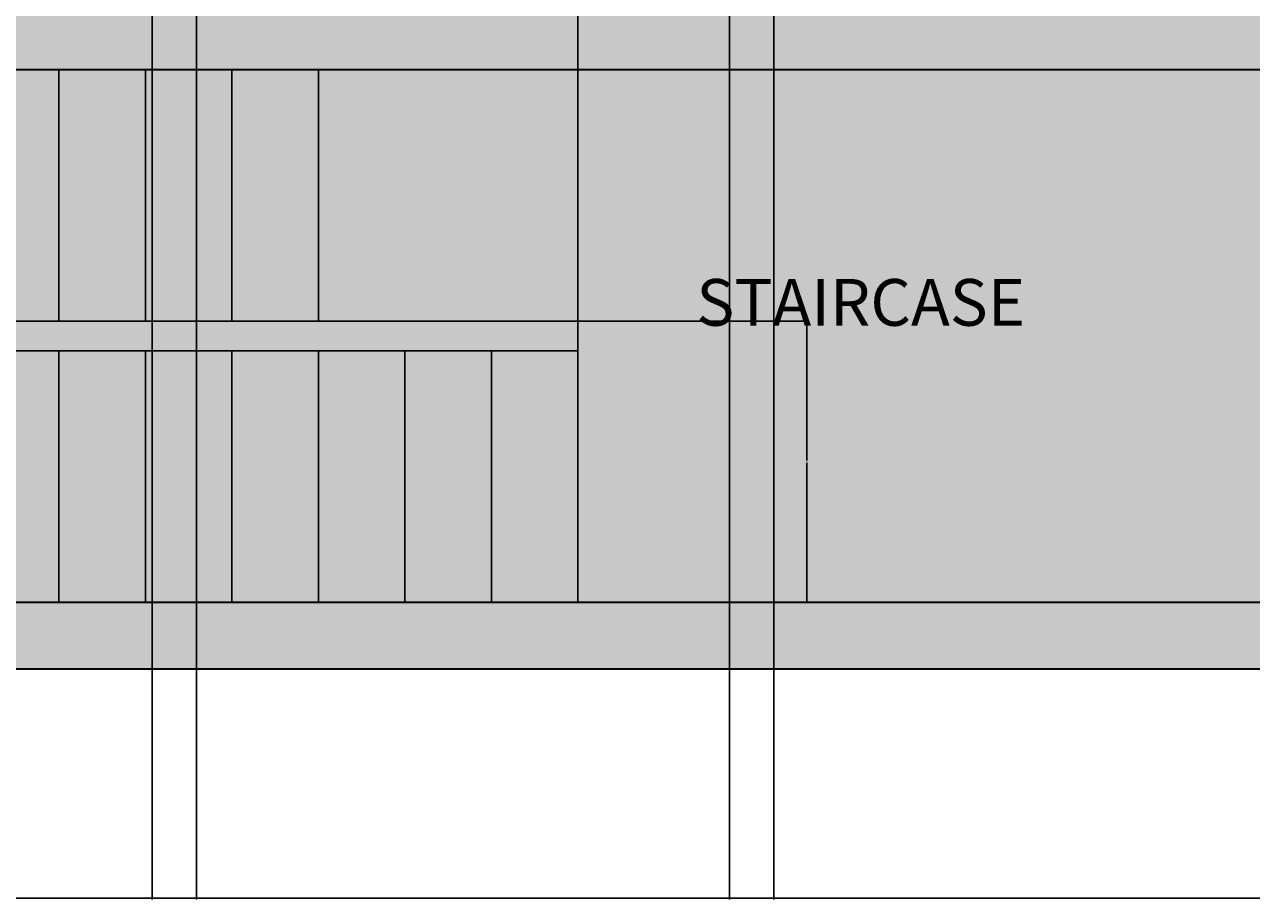
# Model space of a CAD drawing. Units: inches. Extents: x 2549 to 3108, y 1683 to 2362.
# Tile 2 of 30: x 2711 to 2877, y 1683 to 1802. Entities that reach past the tile are written whole.
import ezdxf

# ---------------------------------------------------------------- set-up
doc = ezdxf.new("R2010")
doc.units = ezdxf.units.IN
for name, color, linetype, lineweight in [('A-ANNO-DIMS', 2, 'Continuous', 18), ('A-AREA-IDEN', 7, 'Continuous', 18), ('A-FLOR-STRS', 7, 'Continuous', 25), ('A-FLOR-STRS-PATT', 41, 'Continuous', 13), ('A-FURN-PATT', 9, 'Continuous', 13), ('A-WALL', 7, 'Continuous', 35), ('A-WALL-PATT', 89, 'Continuous', 13), ('C-PROP', 7, 'Continuous', 35)]:
    doc.layers.add(name, color=color, linetype=linetype, lineweight=lineweight)
for name, color, linetype, lineweight, true_color in [('C-PKNG-VEHI-PATT', 251, 'Continuous', 13, 0x636466), ('C-PROP-PATT', 252, 'Continuous', 13, 0x939598), ('C-PVMT-PATT', 9, 'Continuous', 13, 0xc7c8ca)]:
    doc.layers.add(name, color=color, linetype=linetype, lineweight=lineweight, true_color=true_color)
doc.styles.get("Standard").update_dxf_attribs({"font": 'arial.ttf'})
doc.dimstyles.get("Standard").update_dxf_attribs({"dimtxt": 0.18, "dimasz": 0.18, "dimexe": 0.18, "dimexo": 0.0625, "dimgap": 0.09, "dimtad": 0, "dimtih": 1, "dimtoh": 1, "dimdec": 4, "dimzin": 0, "dimdsep": 46, "dimtxsty": 'Standard', "dimcen": 0.09, "dimadec": 0, "dimazin": 0, "dimtfac": 1, "dimtdec": 4, "dimtofl": 0, "dimtmove": 0, "dimatfit": 3, "dimfxl": 1, "dimtolj": 1, "dimtzin": 0, "dimarcsym": 0})

# ---------------------------------------------------------------- blocks, each defined once
blk = doc.blocks.new('*D24')
at = {"layer": 'A-ANNO-DIMS', "color": 0, "lineweight": -2, "transparency": 16777216}
for p, q in [((2596.64, 1714.46), (2596.64, 1683.44)), ((3076.64, 1714.46), (3076.64, 1683.44)), ((2596.82, 1683.62), (2836.35, 1683.62)), ((3076.46, 1683.62), (2836.93, 1683.62))]:
    blk.add_line(p, q, dxfattribs=at)
at = {"layer": 'A-ANNO-DIMS', "color": 0, "transparency": 16777216}
for points in [[(2596.82, 1683.65), (2596.82, 1683.59), (2596.64, 1683.62)], [(3076.46, 1683.65), (3076.46, 1683.59), (3076.64, 1683.62)]]:
    blk.add_solid(points, dxfattribs=at)
at = {"layer": 'Defpoints', "color": 0, "transparency": 16777216}
for p in [(2596.64, 1714.52), (3076.64, 1714.52), (3076.64, 1683.62)]:
    blk.add_point(p, dxfattribs=at)
at = {"layer": 'A-ANNO-DIMS', "color": 0, "transparency": 16777216, "insert": (2836.64, 1683.62), "char_height": 0.18, "attachment_point": 5}
blk.add_mtext('\\A1;480', dxfattribs=at)
blk = doc.blocks.new('*D42')
at = {"layer": 'A-ANNO-DIMS', "color": 0, "lineweight": -2, "transparency": 16777216}
for p, q in [((2638.64, 2080.46), (2638.64, 1683.44)), ((2728.64, 2080.46), (2728.64, 1683.44)), ((2638.82, 1683.62), (2683.42, 1683.62)), ((2728.46, 1683.62), (2683.86, 1683.62))]:
    blk.add_line(p, q, dxfattribs=at)
at = {"layer": 'A-ANNO-DIMS', "color": 0, "transparency": 16777216}
for points in [[(2638.82, 1683.65), (2638.82, 1683.59), (2638.64, 1683.62)], [(2728.46, 1683.65), (2728.46, 1683.59), (2728.64, 1683.62)]]:
    blk.add_solid(points, dxfattribs=at)
at = {"layer": 'Defpoints', "color": 0, "transparency": 16777216}
for p in [(2638.64, 2080.52), (2728.64, 2080.52), (2728.64, 1683.62)]:
    blk.add_point(p, dxfattribs=at)
at = {"layer": 'A-ANNO-DIMS', "color": 0, "transparency": 16777216, "insert": (2683.64, 1683.62), "char_height": 0.18, "attachment_point": 5}
blk.add_mtext('\\A1;90', dxfattribs=at)
blk = doc.blocks.new('*D43')
at = {"layer": 'A-ANNO-DIMS', "color": 0, "lineweight": -2, "transparency": 16777216}
for p, q in [((2734.64, 2080.46), (2734.64, 1683.44)), ((2806.64, 2080.46), (2806.64, 1683.44)), ((2734.82, 1683.62), (2770.43, 1683.62)), ((2806.46, 1683.62), (2770.86, 1683.62))]:
    blk.add_line(p, q, dxfattribs=at)
at = {"layer": 'A-ANNO-DIMS', "color": 0, "transparency": 16777216}
for points in [[(2734.82, 1683.65), (2734.82, 1683.59), (2734.64, 1683.62)], [(2806.46, 1683.65), (2806.46, 1683.59), (2806.64, 1683.62)]]:
    blk.add_solid(points, dxfattribs=at)
at = {"layer": 'Defpoints', "color": 0, "transparency": 16777216}
for p in [(2734.64, 2080.52), (2806.64, 2080.52), (2806.64, 1683.62)]:
    blk.add_point(p, dxfattribs=at)
at = {"layer": 'A-ANNO-DIMS', "color": 0, "transparency": 16777216, "insert": (2770.64, 1683.62), "char_height": 0.18, "attachment_point": 5}
blk.add_mtext('\\A1;72', dxfattribs=at)
blk = doc.blocks.new('*D44')
at = {"layer": 'A-ANNO-DIMS', "color": 0, "lineweight": -2, "transparency": 16777216}
for p, q in [((2662.64, 2040.99), (2662.64, 1683.44)), ((2806.64, 2016.13), (2806.64, 1683.44)), ((2662.82, 1683.62), (2734.36, 1683.62)), ((2806.46, 1683.62), (2734.92, 1683.62))]:
    blk.add_line(p, q, dxfattribs=at)
at = {"layer": 'A-ANNO-DIMS', "color": 0, "transparency": 16777216}
for points in [[(2662.82, 1683.65), (2662.82, 1683.59), (2662.64, 1683.62)], [(2806.46, 1683.65), (2806.46, 1683.59), (2806.64, 1683.62)]]:
    blk.add_solid(points, dxfattribs=at)
at = {"layer": 'Defpoints', "color": 0, "transparency": 16777216}
for p in [(2662.64, 2041.06), (2806.64, 2016.19), (2806.64, 1683.62)]:
    blk.add_point(p, dxfattribs=at)
at = {"layer": 'A-ANNO-DIMS', "color": 0, "transparency": 16777216, "insert": (2734.64, 1683.62), "char_height": 0.18, "attachment_point": 5}
blk.add_mtext('\\A1;144', dxfattribs=at)
blk = doc.blocks.new('*D46')
at = {"layer": 'A-ANNO-DIMS', "color": 0, "lineweight": -2, "transparency": 16777216}
for p, q in [((2812.64, 2140.46), (2812.64, 1683.44)), ((3034.64, 2134.46), (3034.64, 1683.44)), ((2812.82, 1683.62), (2923.35, 1683.62)), ((3034.46, 1683.62), (2923.93, 1683.62))]:
    blk.add_line(p, q, dxfattribs=at)
at = {"layer": 'A-ANNO-DIMS', "color": 0, "transparency": 16777216}
for points in [[(2812.82, 1683.65), (2812.82, 1683.59), (2812.64, 1683.62)], [(3034.46, 1683.65), (3034.46, 1683.59), (3034.64, 1683.62)]]:
    blk.add_solid(points, dxfattribs=at)
at = {"layer": 'Defpoints', "color": 0, "transparency": 16777216}
for p in [(2812.64, 2140.52), (3034.64, 2134.52), (3034.64, 1683.62)]:
    blk.add_point(p, dxfattribs=at)
at = {"layer": 'A-ANNO-DIMS', "color": 0, "transparency": 16777216, "insert": (2923.64, 1683.62), "char_height": 0.18, "attachment_point": 5}
blk.add_mtext('\\A1;222', dxfattribs=at)
blk = doc.blocks.new('*D59')
at = {"layer": 'A-ANNO-DIMS', "color": 0, "lineweight": -2, "transparency": 16777216}
for p, q in [((2680.98, 1761.59), (2680.98, 2362.32)), ((2681.16, 2362.14), (2733.11, 2362.14)), ((2785.98, 2362.14), (2734.02, 2362.14)), ((2786.16, 1761.59), (2786.16, 2362.32))]:
    blk.add_line(p, q, dxfattribs=at)
at = {"layer": 'A-ANNO-DIMS', "color": 0, "transparency": 16777216}
for points in [[(2681.16, 2362.17), (2681.16, 2362.11), (2680.98, 2362.14)], [(2785.98, 2362.17), (2785.98, 2362.11), (2786.16, 2362.14)]]:
    blk.add_solid(points, dxfattribs=at)
at = {"layer": 'Defpoints', "color": 0, "transparency": 16777216}
for p in [(2786.16, 2362.14), (2680.98, 1761.52), (2786.16, 1761.52)]:
    blk.add_point(p, dxfattribs=at)
at = {"layer": 'A-ANNO-DIMS', "color": 0, "transparency": 16777216, "insert": (2733.57, 2362.14), "char_height": 0.18, "attachment_point": 5}
blk.add_mtext('\\A1;105.18', dxfattribs=at)
blk = doc.blocks.new('*D60')
at = {"layer": 'A-ANNO-DIMS', "color": 0, "lineweight": -2, "transparency": 16777216}
for p, q in [((2786.22, 1761.52), (2817.24, 1761.52)), ((2817.06, 1761.34), (2817.06, 1742.71)), ((2817.06, 1723.7), (2817.06, 1742.34)), ((2786.22, 1723.52), (2817.24, 1723.52))]:
    blk.add_line(p, q, dxfattribs=at)
at = {"layer": 'A-ANNO-DIMS', "color": 0, "transparency": 16777216}
for points in [[(2817.03, 1761.34), (2817.09, 1761.34), (2817.06, 1761.52)], [(2817.03, 1723.7), (2817.09, 1723.7), (2817.06, 1723.52)]]:
    blk.add_solid(points, dxfattribs=at)
at = {"layer": 'Defpoints', "color": 0, "transparency": 16777216}
for p in [(2786.16, 1761.52), (2786.16, 1723.52), (2817.06, 1723.52)]:
    blk.add_point(p, dxfattribs=at)
at = {"layer": 'A-ANNO-DIMS', "color": 0, "transparency": 16777216, "insert": (2817.06, 1742.52), "char_height": 0.18, "attachment_point": 5}
blk.add_mtext('\\A1;38', dxfattribs=at)

msp = doc.modelspace()

# ---------------------------------------------------------------- hatches: boundary and pattern name
at = {"layer": 'A-FLOR-STRS-PATT', "transparency": 33554567}
h = msp.add_hatch(color=256, dxfattribs=at)
h.dxf.hatch_style = 1
h.paths.add_polyline_path([(2680.9778, 1795.5237), (2662.6427, 1795.5237), (2638.6427, 1795.5237), (2638.6427, 1723.5237), (2680.9778, 1723.5237)])
h.paths.add_polyline_path([(2692.6645, 1795.5237), (2680.9778, 1795.5237), (2680.9778, 1761.5237), (2692.6645, 1761.5237)])
h.paths.add_polyline_path([(2704.3511, 1795.5237), (2692.6645, 1795.5237), (2692.6645, 1761.5237), (2704.3511, 1761.5237)])
h.paths.add_polyline_path([(2716.0378, 1795.5237), (2704.3511, 1795.5237), (2704.3511, 1761.5237), (2716.0378, 1761.5237)])
h.paths.add_polyline_path([(2727.7244, 1795.5237), (2716.0378, 1795.5237), (2716.0378, 1761.5237), (2727.7244, 1761.5237)])
h.paths.add_polyline_path([(2739.4111, 1795.5237), (2727.7244, 1795.5237), (2727.7244, 1761.5237), (2739.4111, 1761.5237)])
h.paths.add_polyline_path([(2751.0977, 1795.5237), (2739.4111, 1795.5237), (2739.4111, 1761.5237), (2751.0977, 1761.5237)])
h.paths.add_polyline_path([(2786.1577, 1757.5237), (2774.471, 1757.5237), (2774.471, 1723.5237), (2786.1577, 1723.5237)])
h.paths.add_polyline_path([(2774.471, 1757.5237), (2762.7844, 1757.5237), (2762.7844, 1723.5237), (2774.471, 1723.5237)])
h.paths.add_polyline_path([(2762.7844, 1757.5237), (2751.0977, 1757.5237), (2751.0977, 1723.5237), (2762.7844, 1723.5237)])
h.paths.add_polyline_path([(2751.0977, 1757.5237), (2739.4111, 1757.5237), (2739.4111, 1723.5237), (2751.0977, 1723.5237)])
h.paths.add_polyline_path([(2727.7244, 1757.5237), (2716.0378, 1757.5237), (2716.0378, 1723.5237), (2727.7244, 1723.5237)])
h.paths.add_polyline_path([(2716.0378, 1757.5237), (2704.3511, 1757.5237), (2704.3511, 1723.5237), (2716.0378, 1723.5237)])
h.paths.add_polyline_path([(2704.3511, 1757.5237), (2692.6645, 1757.5237), (2692.6645, 1723.5237), (2704.3511, 1723.5237)])
h.paths.add_polyline_path([(2692.6645, 1757.5237), (2680.9778, 1757.5237), (2680.9778, 1723.5237), (2692.6645, 1723.5237)])
h.paths.add_polyline_path([(2739.4111, 1757.5237), (2727.7244, 1757.5237), (2727.7244, 1723.5237), (2739.4111, 1723.5237)])
h.paths.add_polyline_path([(2786.1577, 1761.5237), (2680.9778, 1761.5237), (2680.9778, 1757.5237), (2786.1577, 1757.5237)])
at = {"layer": 'A-FURN-PATT', "transparency": 33554567}
h = msp.add_hatch(color=256, dxfattribs=at)
h.dxf.hatch_style = 1
h.paths.add_polyline_path([(2708.7147, 2271.6737), (2675.2813, 2271.6737), (2675.2813, 2262.0404), (2708.7147, 2262.0404)])
h.paths.add_polyline_path([(2980.8246, 2271.6737), (2947.3913, 2271.6737), (2947.3913, 2262.0404), (2980.8246, 2262.0404)])
h.paths.add_polyline_path([(2748.8496, 2101.6383), (2798.148, 2101.6383), (2798.148, 2111.4248), (2748.8496, 2111.4248)], flags=9)
h.paths.add_polyline_path([(2685.2081, 2101.489), (2719.3253, 2101.489), (2719.3253, 2111.2819), (2685.2081, 2111.2819)], flags=9)
h.paths.add_polyline_path([(2814.6852, 1907.1328), (2847.8384, 1907.1328), (2847.8384, 1916.9258), (2814.6852, 1916.9258)], flags=9)
h.paths.add_polyline_path([(2814.3906, 1835.5864), (2848.0172, 1835.5864), (2848.0172, 1845.3794), (2814.3906, 1845.3794)], flags=9)
h.paths.add_polyline_path([(2800.5245, 1759.1674), (2853.7435, 1759.1674), (2853.7435, 1768.954), (2800.5245, 1768.954)], flags=9)
h.paths.add_polyline_path([(2972.4611, 1807.3305), (3015.3943, 1807.3305), (3015.3943, 1817.117), (2972.4611, 1817.117)], flags=9)
h.paths.add_polyline_path([(2902.3327, 1888.6731), (2937.9131, 1888.6731), (2937.9131, 1898.4661), (2902.3327, 1898.4661)], flags=9)
h.paths.add_polyline_path([(2712.1779, 1878.9039), (2754.1257, 1878.9039), (2754.1257, 1888.6904), (2712.1779, 1888.6904)], flags=9)
h.paths.add_polyline_path([(2614.0056, 2012.812), (2650.0251, 2012.812), (2650.0251, 2022.4371), (2614.0056, 2022.4371)], flags=9)
h.paths.add_polyline_path([(2713.3129, 2003.1645), (2747.4237, 2003.1645), (2747.4237, 2012.951), (2713.3129, 2012.951)], flags=9)
h.paths.add_polyline_path([(2950.1379, 2001.6934), (2982.2992, 2001.6934), (2982.2992, 2011.48), (2950.1379, 2011.48)], flags=9)
h.paths.add_polyline_path([(2940.864, 2238.5537), (2997.5066, 2238.5537), (2997.5066, 2248.3466), (2940.864, 2248.3466)], flags=9)
h.paths.add_polyline_path([(2821.5457, 2202.8348), (2855.663, 2202.8348), (2855.663, 2212.6278), (2821.5457, 2212.6278)], flags=9)
h.paths.add_polyline_path([(2661.8026, 2238.6249), (2718.4451, 2238.6249), (2718.4451, 2248.4179), (2661.8026, 2248.4179)], flags=9)
h = msp.add_hatch(color=256, dxfattribs=at)
h.dxf.hatch_style = 1
h.paths.add_polyline_path([(2906.5064, 1905.2148), (2905.2584, 1904.3827), (2907.0611, 1900.7772), (2908.3092, 1901.6092)])
h.paths.add_polyline_path([(2936.522, 1914.8044), (2935.2739, 1915.6364), (2932.6391, 1912.5856), (2933.8871, 1911.7535)])
h.paths.add_polyline_path([(2950.2508, 1905.6518), (2949.0027, 1906.4839), (2947.1999, 1902.8783), (2948.448, 1902.0463)])
h.paths.add_polyline_path([(2958.5713, 1918.1326), (2956.9072, 1919.242), (2952.4696, 1908.98, 1.38742744), (2954.9657, 1907.3159)])
h.paths.add_polyline_path([(2945.2585, 1927.0078), (2943.5944, 1928.1172), (2934.9965, 1920.6287, 1.38742744), (2937.4927, 1918.9646)])
h.paths.add_polyline_path([(2748.8496, 2101.6383), (2798.148, 2101.6383), (2798.148, 2111.4248), (2748.8496, 2111.4248)], flags=9)
h.paths.add_polyline_path([(2685.2081, 2101.489), (2719.3253, 2101.489), (2719.3253, 2111.2819), (2685.2081, 2111.2819)], flags=9)
h.paths.add_polyline_path([(2814.6852, 1907.1328), (2847.8384, 1907.1328), (2847.8384, 1916.9258), (2814.6852, 1916.9258)], flags=9)
h.paths.add_polyline_path([(2814.3906, 1835.5864), (2848.0172, 1835.5864), (2848.0172, 1845.3794), (2814.3906, 1845.3794)], flags=9)
h.paths.add_polyline_path([(2800.5245, 1759.1674), (2853.7435, 1759.1674), (2853.7435, 1768.954), (2800.5245, 1768.954)], flags=9)
h.paths.add_polyline_path([(2972.4611, 1807.3305), (3015.3943, 1807.3305), (3015.3943, 1817.117), (2972.4611, 1817.117)], flags=9)
h.paths.add_polyline_path([(2902.3327, 1888.6731), (2937.9131, 1888.6731), (2937.9131, 1898.4661), (2902.3327, 1898.4661)], flags=9)
h.paths.add_polyline_path([(2712.1779, 1878.9039), (2754.1257, 1878.9039), (2754.1257, 1888.6904), (2712.1779, 1888.6904)], flags=9)
h.paths.add_polyline_path([(2614.0056, 2012.812), (2650.0251, 2012.812), (2650.0251, 2022.4371), (2614.0056, 2022.4371)], flags=9)
h.paths.add_polyline_path([(2713.3129, 2003.1645), (2747.4237, 2003.1645), (2747.4237, 2012.951), (2713.3129, 2012.951)], flags=9)
h.paths.add_polyline_path([(2950.1379, 2001.6934), (2982.2992, 2001.6934), (2982.2992, 2011.48), (2950.1379, 2011.48)], flags=9)
h.paths.add_polyline_path([(2940.864, 2238.5537), (2997.5066, 2238.5537), (2997.5066, 2248.3466), (2940.864, 2248.3466)], flags=9)
h.paths.add_polyline_path([(2821.5457, 2202.8348), (2855.663, 2202.8348), (2855.663, 2212.6278), (2821.5457, 2212.6278)], flags=9)
h.paths.add_polyline_path([(2661.8026, 2238.6249), (2718.4451, 2238.6249), (2718.4451, 2248.4179), (2661.8026, 2248.4179)], flags=9)
at = {"layer": 'A-WALL-PATT'}
h = msp.add_hatch(color=256, dxfattribs=at)
h.dxf.hatch_style = 1
h.paths.add_polyline_path([(2638.6427, 2272.5237), (3034.6427, 2272.5237), (3034.6427, 1936.5237), (3043.6427, 1936.5237), (3043.6427, 2281.5237), (2629.6427, 2281.5237), (2629.6427, 2074.5237), (2812.6427, 2074.5237), (2812.6427, 2140.5237), (2785.7177, 2140.5237), (2785.7177, 2134.5237), (2806.6427, 2134.5237), (2806.6427, 2080.5237), (2638.6427, 2080.5237)])
h.paths.add_polyline_path([(2638.6427, 1972.5237), (2662.6427, 1972.5237), (2662.6427, 2041.0557), (2653.6427, 2041.0557), (2653.6427, 1978.5237), (2629.6427, 1978.5237), (2629.6427, 1795.5237), (2662.6427, 1795.5237), (2881.6427, 1795.5237), (2881.6427, 1936.5237), (2965.9351, 1936.5237), (2965.9351, 1974.5439), (2959.9351, 1974.5439), (2959.9351, 1945.5237), (2881.6427, 1945.5237), (2872.6427, 1945.5237), (2872.6427, 1804.5237), (2662.6427, 1804.5237), (2638.6427, 1804.5237)])
at = {"layer": 'C-PKNG-VEHI-PATT'}
h = msp.add_hatch(color=256, dxfattribs=at)
h.dxf.hatch_style = 1
edge = h.paths.add_edge_path()
edge.add_ellipse((2935.7258, 1791.964), major_axis=(-50.66, 0), ratio=0.84230387, start_angle=248.165046, end_angle=265.722579)
edge.add_line((2938.911, 1834.5507), (2925.8653, 1834.5507))
edge.add_ellipse((2929.0505, 1791.964), major_axis=(50.66, 0), ratio=0.84230387, start_angle=94.277421, end_angle=111.834954)
edge.add_line((2912.8508, 1832.3947), (2914.2044, 1822.2495))
edge.add_ellipse((2930.6538, 1783.1023), major_axis=(-49.3014, 0), ratio=0.84230387, start_angle=-85.12993, end_angle=-67.208085, ccw=False)
edge.add_line((2927.1247, 1824.5225), (2937.6516, 1824.5225))
edge.add_ellipse((2934.1225, 1783.1023), major_axis=(49.3014, 0), ratio=0.84230387, start_angle=67.208085, end_angle=85.12993, ccw=False)
edge.add_line((2950.5719, 1822.2495), (2951.9255, 1832.3947))
edge = h.paths.add_edge_path()
edge.add_ellipse((2903.4793, 1857.3351), major_axis=(-34.7979, 0), ratio=0.84230387, start_angle=180, end_angle=209.43857)
edge.add_ellipse((2961.297, 1857.3351), major_axis=(34.7979, 0), ratio=0.84230387, start_angle=150.56143, end_angle=180)
edge.add_line((2926.4991, 1857.3351), (2926.4991, 1843.7609))
edge.add_ellipse((2924.1251, 1844.3143), major_axis=(-0.2209, 3.9278), ratio=0.60383358, start_angle=89.002014, end_angle=253.657408, ccw=False)
edge.add_line((2921.7512, 1844.2222), (2921.7512, 1853.3975))
edge.add_line((2921.7512, 1853.3975), (2925.269, 1855.8484))
edge.add_ellipse((2925.4782, 1855.4931), major_axis=(0.4584, 0), ratio=0.84230387, start_angle=90, end_angle=134.480211, ccw=False)
edge.add_line((2925.4782, 1855.8792), (2926.4991, 1855.8792))
edge.add_line((2926.4991, 1855.8792), (2926.4991, 1857.3351))
edge.add_ellipse((2961.297, 1857.3351), major_axis=(34.7979, 0), ratio=0.84230387, start_angle=150.56143, end_angle=180, ccw=False)
edge.add_line((2932.3882, 1873.6501), (2932.3882, 1875.7801))
edge.add_ellipse((2932.3882, 1875.3939), major_axis=(0.4584, 0), ratio=0.84230387, start_angle=90, end_angle=127.93313)
edge.add_line((2932.1366, 1875.7167), (2928.5915, 1873.7564))
edge.add_ellipse((2899.9271, 2002.4692), major_axis=(155.4756, 0), ratio=0.84230387, start_angle=-80.743434, end_angle=-77.445067, ccw=False)
edge.add_ellipse((2949.4402, 1715.2151), major_axis=(-189.1422, 0), ratio=0.84230387, start_angle=-79.790461, end_angle=-77.555373)
edge.add_ellipse((3300.3614, 1852.5642), major_axis=(-386.1662, 0), ratio=0.84230387, start_angle=-2.863715, end_angle=2.198541)
edge.add_ellipse((2929.0505, 1792.5159), major_axis=(-55.6192, 0), ratio=0.84230387, start_angle=-85.917589, end_angle=-72.280047, ccw=False)
edge.add_line((2925.7129, 1839.2798), (2939.0634, 1839.2798))
edge.add_ellipse((2935.7258, 1792.5159), major_axis=(55.6192, 0), ratio=0.84230387, start_angle=72.280047, end_angle=85.917589, ccw=False)
edge.add_ellipse((2564.4149, 1852.5642), major_axis=(-386.1662, 0), ratio=0.84230387, start_angle=177.801459, end_angle=182.863715)
edge.add_ellipse((2915.3361, 1715.2151), major_axis=(189.1422, 0), ratio=0.84230387, start_angle=77.555373, end_angle=79.790461)
edge.add_ellipse((2964.8492, 2002.4692), major_axis=(-155.4756, 0), ratio=0.84230387, start_angle=77.445067, end_angle=80.743434, ccw=False)
edge.add_line((2936.1848, 1873.7564), (2932.6397, 1875.7167))
edge.add_ellipse((2932.3882, 1875.3939), major_axis=(0.4584, 0), ratio=0.84230387, start_angle=52.06687, end_angle=90)
edge.add_line((2932.3882, 1875.7801), (2932.3882, 1873.6501))
edge.add_ellipse((2903.4793, 1857.3351), major_axis=(-34.7979, 0), ratio=0.84230387, start_angle=180, end_angle=209.43857, ccw=False)
edge.add_line((2938.2772, 1857.3351), (2938.2772, 1855.8792))
edge.add_line((2938.2772, 1855.8792), (2939.4059, 1855.8792))
edge.add_ellipse((2939.2981, 1855.4931), major_axis=(-0.4584, 0), ratio=0.84230387, start_angle=225.519789, end_angle=270, ccw=False)
edge.add_line((2939.5903, 1855.7906), (2943.0251, 1853.3975))
edge.add_line((2943.0251, 1853.3975), (2943.0251, 1844.2222))
edge.add_ellipse((2940.6512, 1844.3143), major_axis=(0.2209, 3.9278), ratio=0.60383358, start_angle=106.342592, end_angle=270.997986, ccw=False)
edge.add_line((2938.2772, 1843.7609), (2938.2772, 1857.3351))
edge = h.paths.add_edge_path()
edge.add_ellipse((2932.3882, 1865.1973), major_axis=(91.081, 0), ratio=0.84230387, start_angle=256.401865, end_angle=283.598135, ccw=False)
edge.add_line((2914.2044, 1790.0239), (2914.2044, 1778.3622))
edge.add_ellipse((2932.3882, 1853.5356), major_axis=(91.081, 0), ratio=0.84230387, start_angle=256.401865, end_angle=283.598135)
edge.add_line((2950.5719, 1778.3622), (2950.5719, 1790.0239))
edge = h.paths.add_edge_path()
edge.add_ellipse((2948.7383, 1772.3145), major_axis=(1.8336, 0), ratio=0.84230387, start_angle=0, end_angle=90)
edge.add_line((2948.7383, 1773.859), (2916.038, 1773.859))
edge.add_ellipse((2916.038, 1772.3145), major_axis=(1.8336, 0), ratio=0.84230387, start_angle=90, end_angle=180)
edge.add_line((2914.2044, 1772.3145), (2914.2044, 1760.2558))
edge.add_line((2914.2044, 1760.2558), (2950.5719, 1760.2558))
edge.add_line((2950.5719, 1760.2558), (2950.5719, 1772.3145))
h.paths.add_polyline_path([(2748.8496, 2101.6383), (2798.148, 2101.6383), (2798.148, 2111.4248), (2748.8496, 2111.4248)], flags=9)
h.paths.add_polyline_path([(2685.2081, 2101.489), (2719.3253, 2101.489), (2719.3253, 2111.2819), (2685.2081, 2111.2819)], flags=9)
h.paths.add_polyline_path([(2814.6852, 1907.1328), (2847.8384, 1907.1328), (2847.8384, 1916.9258), (2814.6852, 1916.9258)], flags=9)
h.paths.add_polyline_path([(2814.3906, 1835.5864), (2848.0172, 1835.5864), (2848.0172, 1845.3794), (2814.3906, 1845.3794)], flags=9)
h.paths.add_polyline_path([(2800.5245, 1759.1674), (2853.7435, 1759.1674), (2853.7435, 1768.954), (2800.5245, 1768.954)], flags=9)
h.paths.add_polyline_path([(2972.4611, 1807.3305), (3015.3943, 1807.3305), (3015.3943, 1817.117), (2972.4611, 1817.117)], flags=9)
h.paths.add_polyline_path([(2902.3327, 1888.6731), (2937.9131, 1888.6731), (2937.9131, 1898.4661), (2902.3327, 1898.4661)], flags=9)
h.paths.add_polyline_path([(2712.1779, 1878.9039), (2754.1257, 1878.9039), (2754.1257, 1888.6904), (2712.1779, 1888.6904)], flags=9)
h.paths.add_polyline_path([(2614.0056, 2012.812), (2650.0251, 2012.812), (2650.0251, 2022.4371), (2614.0056, 2022.4371)], flags=9)
h.paths.add_polyline_path([(2713.3129, 2003.1645), (2747.4237, 2003.1645), (2747.4237, 2012.951), (2713.3129, 2012.951)], flags=9)
h.paths.add_polyline_path([(2950.1379, 2001.6934), (2982.2992, 2001.6934), (2982.2992, 2011.48), (2950.1379, 2011.48)], flags=9)
h.paths.add_polyline_path([(2940.864, 2238.5537), (2997.5066, 2238.5537), (2997.5066, 2248.3466), (2940.864, 2248.3466)], flags=9)
h.paths.add_polyline_path([(2821.5457, 2202.8348), (2855.663, 2202.8348), (2855.663, 2212.6278), (2821.5457, 2212.6278)], flags=9)
h.paths.add_polyline_path([(2661.8026, 2238.6249), (2718.4451, 2238.6249), (2718.4451, 2248.4179), (2661.8026, 2248.4179)], flags=9)
at = {"layer": 'C-PROP-PATT'}
h = msp.add_hatch(color=256, dxfattribs=at)
h.dxf.hatch_style = 1
h.paths.add_polyline_path([(3076.6427, 2314.5237), (2596.6427, 2314.5237), (2596.6427, 1714.5237), (2881.84, 1714.5237), (2881.84, 1723.5237), (2605.6427, 1723.5237), (2605.6427, 2305.5237), (3067.6427, 2305.5237), (3067.6427, 1723.5237), (3067.6427, 1714.5237), (3076.6427, 1714.5237)])
at = {"layer": 'C-PVMT-PATT'}
h = msp.add_hatch(color=256, dxfattribs=at)
h.dxf.hatch_style = 1
h.paths.add_polyline_path([(3067.6427, 2305.5237), (2605.6427, 2305.5237), (2605.6427, 2074.5237), (2629.6427, 2074.5237), (2629.6427, 2281.5237), (3043.6427, 2281.5237), (3043.6427, 1885.5237), (3043.6427, 1872.8745), (3031.1672, 1872.8745), (3031.1672, 1862.5731), (2995.8054, 1862.5731), (2995.8054, 1872.8745), (2983.1752, 1872.8745), (2983.1752, 1885.5237), (2881.6427, 1885.5237), (2881.6427, 1795.5237), (2751.0977, 1795.5237), (2751.0977, 1761.5237), (2786.1577, 1761.5237), (2786.1577, 1723.5237), (2881.84, 1723.5237), (2881.84, 1714.5237), (3067.6427, 1714.5237), (3067.6427, 1723.5237)])
edge = h.paths.add_edge_path(flags=16)
edge.add_ellipse((2949.4402, 1710.9683), major_axis=(-194.1014, 0), ratio=0.84230387, start_angle=-77.874034, end_angle=-76.219471, ccw=False)
edge.add_ellipse((2949.4402, 1715.2151), major_axis=(-189.1422, 0), ratio=0.84230387, start_angle=-79.790461, end_angle=-77.555373, ccw=False)
edge.add_ellipse((2899.9271, 2002.4692), major_axis=(155.4756, 0), ratio=0.84230387, start_angle=-80.743434, end_angle=-77.445067)
edge.add_line((2928.5915, 1873.7564), (2932.3882, 1875.8558))
edge.add_line((2932.3882, 1875.8558), (2936.1848, 1873.7564))
edge.add_ellipse((2964.8492, 2002.4692), major_axis=(-155.4756, 0), ratio=0.84230387, start_angle=77.445067, end_angle=80.743434)
edge.add_ellipse((2915.3361, 1715.2151), major_axis=(189.1422, 0), ratio=0.84230387, start_angle=77.555373, end_angle=79.790461, ccw=False)
edge.add_ellipse((2915.3361, 1710.9683), major_axis=(-194.1014, 0), ratio=0.84230387, start_angle=256.219471, end_angle=257.874034, ccw=False)
edge.add_ellipse((2628.2871, 1850.2612), major_axis=(-327.2532, 0), ratio=0.84230387, start_angle=182.17995, end_angle=183.650428, ccw=False)
edge.add_ellipse((2955.5637, 1861.9334), major_axis=(-0.9168, 0), ratio=0.84230387, start_angle=180, end_angle=270, ccw=False)
edge.add_line((2956.4805, 1862.3857), (2956.4805, 1846.4866))
edge.add_ellipse((2955.5637, 1846.939), major_axis=(-0.9168, 0), ratio=0.84230387, start_angle=90, end_angle=180, ccw=False)
edge.add_ellipse((-3607.0606, 1835.832), major_axis=(-6562.6242, 0), ratio=0.84230387, start_angle=179.61613322, end_angle=180.09022909, ccw=False)
edge.add_ellipse((2955.5637, 1791.0926), major_axis=(0.9168, 0), ratio=0.84230387, start_angle=0, end_angle=90, ccw=False)
edge.add_line((2956.4805, 1791.545), (2956.4805, 1775.6459))
edge.add_ellipse((2955.5637, 1776.0982), major_axis=(0.9168, 0), ratio=0.84230387, start_angle=270, end_angle=360, ccw=False)
edge.add_ellipse((-3607.0606, 1835.832), major_axis=(-6562.6242, 0), ratio=0.84230387, start_angle=179.3813568, end_angle=179.47172853, ccw=False)
edge.add_ellipse((2954.5907, 1763.8768), major_axis=(-1.3752, 0), ratio=0.84230387, start_angle=179.371763, end_angle=248.464757, ccw=False)
edge.add_ellipse((-3607.519, 1835.832), major_axis=(-6564.0409, 0), ratio=0.842303863, start_angle=179.35344594, end_angle=179.37176282, ccw=False)
edge.add_ellipse((2952.6829, 1761.8002), major_axis=(3.2503, 0), ratio=0.84230387, start_angle=-90, end_angle=-0.646554, ccw=False)
edge.add_line((2952.6829, 1759.0625), (2912.0934, 1759.0625))
edge.add_ellipse((2912.0934, 1761.8002), major_axis=(3.2503, 0), ratio=0.84230387, start_angle=180.646554, end_angle=270, ccw=False)
edge.add_ellipse((9472.2953, 1835.832), major_axis=(-6564.0409, 0), ratio=0.842303871, start_angle=0.62823722, end_angle=0.6465541, ccw=False)
edge.add_ellipse((2910.1856, 1763.8768), major_axis=(1.3752, 0), ratio=0.84230387, start_angle=111.535244, end_angle=180.628237, ccw=False)
edge.add_ellipse((9471.8369, 1835.832), major_axis=(-6562.6242, 0), ratio=0.84230387, start_angle=0.52827147, end_angle=0.6465541, ccw=False)
edge.add_ellipse((2909.2126, 1776.0982), major_axis=(-0.9168, 0), ratio=0.84230387, start_angle=0, end_angle=90, ccw=False)
edge.add_line((2908.2958, 1775.6459), (2908.2958, 1791.545))
edge.add_ellipse((2909.2126, 1791.0926), major_axis=(-0.9168, 0), ratio=0.84230387, start_angle=-90, end_angle=0, ccw=False)
edge.add_ellipse((9471.8369, 1835.832), major_axis=(-6562.6242, 0), ratio=0.84230387, start_angle=-0.09022909, end_angle=0.38386678, ccw=False)
edge.add_ellipse((2909.2126, 1846.939), major_axis=(-0.9168, 0), ratio=0.84230387, start_angle=0, end_angle=90, ccw=False)
edge.add_line((2908.2958, 1846.4866), (2908.2958, 1862.3857))
edge.add_ellipse((2909.2126, 1861.9334), major_axis=(0.9168, 0), ratio=0.84230387, start_angle=90, end_angle=180, ccw=False)
edge.add_ellipse((3236.4892, 1850.2612), major_axis=(327.2532, 0), ratio=0.84230387, start_angle=176.349572, end_angle=177.82005, ccw=False)
edge = h.paths.add_edge_path(flags=0)
edge.add_ellipse((2903.4793, 1857.3351), major_axis=(-34.7979, 0), ratio=0.84230387, start_angle=180, end_angle=209.43857, ccw=False)
edge.add_line((2938.2772, 1857.3351), (2938.2772, 1855.8792))
edge.add_line((2938.2772, 1855.8792), (2939.4631, 1855.8792))
edge.add_line((2939.4631, 1855.8792), (2943.0251, 1853.3975))
edge.add_line((2943.0251, 1853.3975), (2943.0251, 1844.2222))
edge.add_ellipse((2940.6512, 1844.3143), major_axis=(0.2209, 3.9278), ratio=0.60383358, start_angle=106.342592, end_angle=270.997986, ccw=False)
edge.add_line((2938.2772, 1843.7609), (2938.2772, 1857.3351))
edge.add_ellipse((2903.4793, 1857.3351), major_axis=(-34.7979, 0), ratio=0.84230387, start_angle=180, end_angle=209.43857)
edge.add_ellipse((2961.297, 1857.3351), major_axis=(34.7979, 0), ratio=0.84230387, start_angle=150.56143, end_angle=180)
edge.add_line((2926.4991, 1857.3351), (2926.4991, 1843.7609))
edge.add_ellipse((2924.1251, 1844.3143), major_axis=(-0.2209, 3.9278), ratio=0.60383358, start_angle=89.002014, end_angle=253.657408, ccw=False)
edge.add_line((2921.7512, 1844.2222), (2921.7512, 1853.3975))
edge.add_line((2921.7512, 1853.3975), (2925.3132, 1855.8792))
edge.add_line((2925.3132, 1855.8792), (2926.4991, 1855.8792))
edge.add_line((2926.4991, 1855.8792), (2926.4991, 1857.3351))
edge.add_ellipse((2961.297, 1857.3351), major_axis=(34.7979, 0), ratio=0.84230387, start_angle=150.56143, end_angle=180, ccw=False)
edge = h.paths.add_edge_path(flags=0)
edge.add_ellipse((2929.0505, 1791.964), major_axis=(50.66, 0), ratio=0.84230387, start_angle=94.277421, end_angle=111.834954, ccw=False)
edge.add_line((2925.8653, 1834.5507), (2938.911, 1834.5507))
edge.add_ellipse((2935.7258, 1791.964), major_axis=(-50.66, 0), ratio=0.84230387, start_angle=248.165046, end_angle=265.722579, ccw=False)
edge.add_line((2951.9255, 1832.3947), (2950.5719, 1822.2495))
edge.add_ellipse((2934.1225, 1783.1023), major_axis=(49.3014, 0), ratio=0.84230387, start_angle=67.208085, end_angle=85.12993)
edge.add_line((2937.6516, 1824.5225), (2927.1247, 1824.5225))
edge.add_ellipse((2930.6538, 1783.1023), major_axis=(-49.3014, 0), ratio=0.84230387, start_angle=-85.12993, end_angle=-67.208085)
edge.add_line((2914.2044, 1822.2495), (2912.8508, 1832.3947))
edge = h.paths.add_edge_path(flags=0)
edge.add_line((2910.1338, 1829.4651), (2912.6432, 1821.2711))
edge.add_ellipse((5203.7787, 1816.4367), major_axis=(-2291.1426, 0), ratio=0.84230387, start_angle=-0.1208974, end_angle=0.3640763)
edge.add_line((2912.7012, 1801.8782), (2910.3305, 1792.5698))
edge.add_ellipse((9471.8369, 1835.832), major_axis=(-6561.7074, 0), ratio=0.84230387, start_angle=0.05559431, end_angle=0.37776419, ccw=False)
edge = h.paths.add_edge_path(flags=0)
edge.add_ellipse((-3607.0606, 1835.832), major_axis=(6561.7074, 0), ratio=0.84230387, start_angle=-0.37776419, end_angle=-0.05559431, ccw=False)
edge.add_line((2954.4458, 1792.5698), (2952.0751, 1801.8782))
edge.add_ellipse((660.9976, 1816.4367), major_axis=(2291.1426, 0), ratio=0.84230387, start_angle=-0.3640763, end_angle=0.1208974)
edge.add_line((2952.1331, 1821.2711), (2954.6425, 1829.4651))
edge = h.paths.add_edge_path(flags=0)
edge.add_ellipse((2932.3882, 1865.1973), major_axis=(91.081, 0), ratio=0.84230387, start_angle=256.401865, end_angle=283.598135)
edge.add_line((2950.5719, 1790.0239), (2950.5719, 1778.3622))
edge.add_ellipse((2932.3882, 1853.5356), major_axis=(91.081, 0), ratio=0.84230387, start_angle=256.401865, end_angle=283.598135, ccw=False)
edge.add_line((2914.2044, 1778.3622), (2914.2044, 1790.0239))
edge = h.paths.add_edge_path(flags=0)
edge.add_line((2916.038, 1773.859), (2948.7383, 1773.859))
edge.add_ellipse((2948.7383, 1772.3145), major_axis=(1.8336, 0), ratio=0.84230387, start_angle=0, end_angle=90, ccw=False)
edge.add_line((2950.5719, 1772.3145), (2950.5719, 1760.2558))
edge.add_line((2950.5719, 1760.2558), (2914.2044, 1760.2558))
edge.add_line((2914.2044, 1760.2558), (2914.2044, 1772.3145))
edge.add_ellipse((2916.038, 1772.3145), major_axis=(1.8336, 0), ratio=0.84230387, start_angle=90, end_angle=180, ccw=False)
h.paths.add_polyline_path([(2629.6427, 1978.5237), (2605.6427, 1978.5237), (2605.6427, 1723.5237), (2629.6427, 1723.5237), (2629.6427, 1795.5237)], flags=17)
h.paths.add_polyline_path([(2800.5245, 1759.1674), (2853.7435, 1759.1674), (2853.7435, 1768.954), (2800.5245, 1768.954)], flags=24)
h.paths.add_polyline_path([(2972.4611, 1807.3305), (3015.3943, 1807.3305), (3015.3943, 1817.117), (2972.4611, 1817.117)], flags=24)

# ---------------------------------------------------------------- linework, layer by layer
at = {"layer": 'A-FLOR-STRS'}
for p, q in [((2716.0378, 1795.5237), (2716.0378, 1761.5237)), ((2727.7244, 1795.5237), (2727.7244, 1761.5237)), ((2739.4111, 1795.5237), (2739.4111, 1761.5237)), ((2751.0977, 1795.5237), (2751.0977, 1761.5237)), ((2786.1577, 1761.5237), (2680.9778, 1761.5237)), ((2786.1577, 1761.5237), (2786.1577, 1723.5237)), ((2786.1577, 1757.5237), (2680.9778, 1757.5237)), ((2716.0378, 1757.5237), (2716.0378, 1723.5237)), ((2727.7244, 1757.5237), (2727.7244, 1723.5237)), ((2739.4111, 1757.5237), (2739.4111, 1723.5237)), ((2751.0977, 1757.5237), (2751.0977, 1723.5237)), ((2762.7844, 1757.5237), (2762.7844, 1723.5237)), ((2774.471, 1757.5237), (2774.471, 1723.5237))]:
    msp.add_line(p, q, dxfattribs=at)
at = {"layer": 'A-WALL'}
msp.add_lwpolyline([(2629.6427, 1795.5237), (2662.6427, 1795.5237), (2881.6427, 1795.5237)], dxfattribs=at)
at = {"layer": 'C-PROP'}
msp.add_lwpolyline([(2596.6427, 2314.5237), (3076.6427, 2314.5237), (3076.6427, 1714.5237), (2596.6427, 1714.5237)], close=True, dxfattribs=at)
msp.add_lwpolyline([(2881.84, 1723.5237), (2605.6427, 1723.5237), (2605.6427, 2305.5237), (3067.6427, 2305.5237), (3067.6427, 1723.5237)], dxfattribs=at)

# ---------------------------------------------------------------- texts
at = {"layer": 'A-AREA-IDEN'}
msp.add_text('STAIRCASE', height=6.30916, dxfattribs=at).set_placement((2802.1555, 1760.9061))

# ---------------------------------------------------------------- dimensions: what is measured, and where the dimension line sits
at = {"layer": 'A-ANNO-DIMS'}
for base, p1, p2, override, picture, middle in [((2786.1577, 2362.1425), (2680.9778, 1761.5237), (2786.1577, 1761.5237), {"dimdec": 2, "dimlfac": 1, "dimrnd": 0, "dimzin": 0, "dimdsep": 46, "dimlunit": 2}, '*D59', (2733.5678, 2362.1425)), ((3034.6427, 1683.6237), (2812.6427, 2140.5237), (3034.6427, 2134.5237), {"dimdec": 0, "dimlfac": 1, "dimrnd": 0, "dimzin": 0, "dimdsep": 46, "dimlunit": 2}, '*D46', (2923.6427, 1683.6237)), ((2728.6427, 1683.6237), (2638.6427, 2080.5237), (2728.6427, 2080.5237), {"dimdec": 0, "dimlfac": 1, "dimrnd": 0, "dimzin": 0, "dimdsep": 46, "dimlunit": 2}, '*D42', (2683.6427, 1683.6237)), ((2806.6427, 1683.6237), (2734.6427, 2080.5237), (2806.6427, 2080.5237), {"dimdec": 0, "dimlfac": 1, "dimrnd": 0, "dimzin": 0, "dimdsep": 46, "dimlunit": 2}, '*D43', (2770.6427, 1683.6237)), ((2806.6427, 1683.6237), (2662.6427, 2041.0557), (2806.6427, 2016.1911), {"dimdec": 0, "dimlfac": 1, "dimrnd": 0, "dimzin": 0, "dimdsep": 46, "dimlunit": 2}, '*D44', (2734.6427, 1683.6237)), ((3076.6427, 1683.6237), (2596.6427, 1714.5237), (3076.6427, 1714.5237), {"dimdec": 0, "dimlfac": 1, "dimrnd": 0, "dimzin": 0, "dimdsep": 46, "dimlunit": 2}, '*D24', (2836.6427, 1683.6237))]:
    dim = msp.add_linear_dim(base=base, p1=p1, p2=p2, dimstyle='Standard', override=override, dxfattribs=at)
    dim.commit()
    dim.dimension.update_dxf_attribs({"geometry": picture, "text_midpoint": middle})
dim = msp.add_linear_dim(base=(2817.0577, 1723.5237), p1=(2786.1577, 1761.5237), p2=(2786.1577, 1723.5237), angle=270, dimstyle='Standard', override={"dimdec": 0, "dimlfac": 1, "dimrnd": 0, "dimzin": 0, "dimdsep": 46, "dimlunit": 2}, dxfattribs=at)
dim.commit()
dim.dimension.update_dxf_attribs({"geometry": '*D60', "text_midpoint": (2817.0577, 1742.5237)})

doc.saveas('drawing.dxf')
